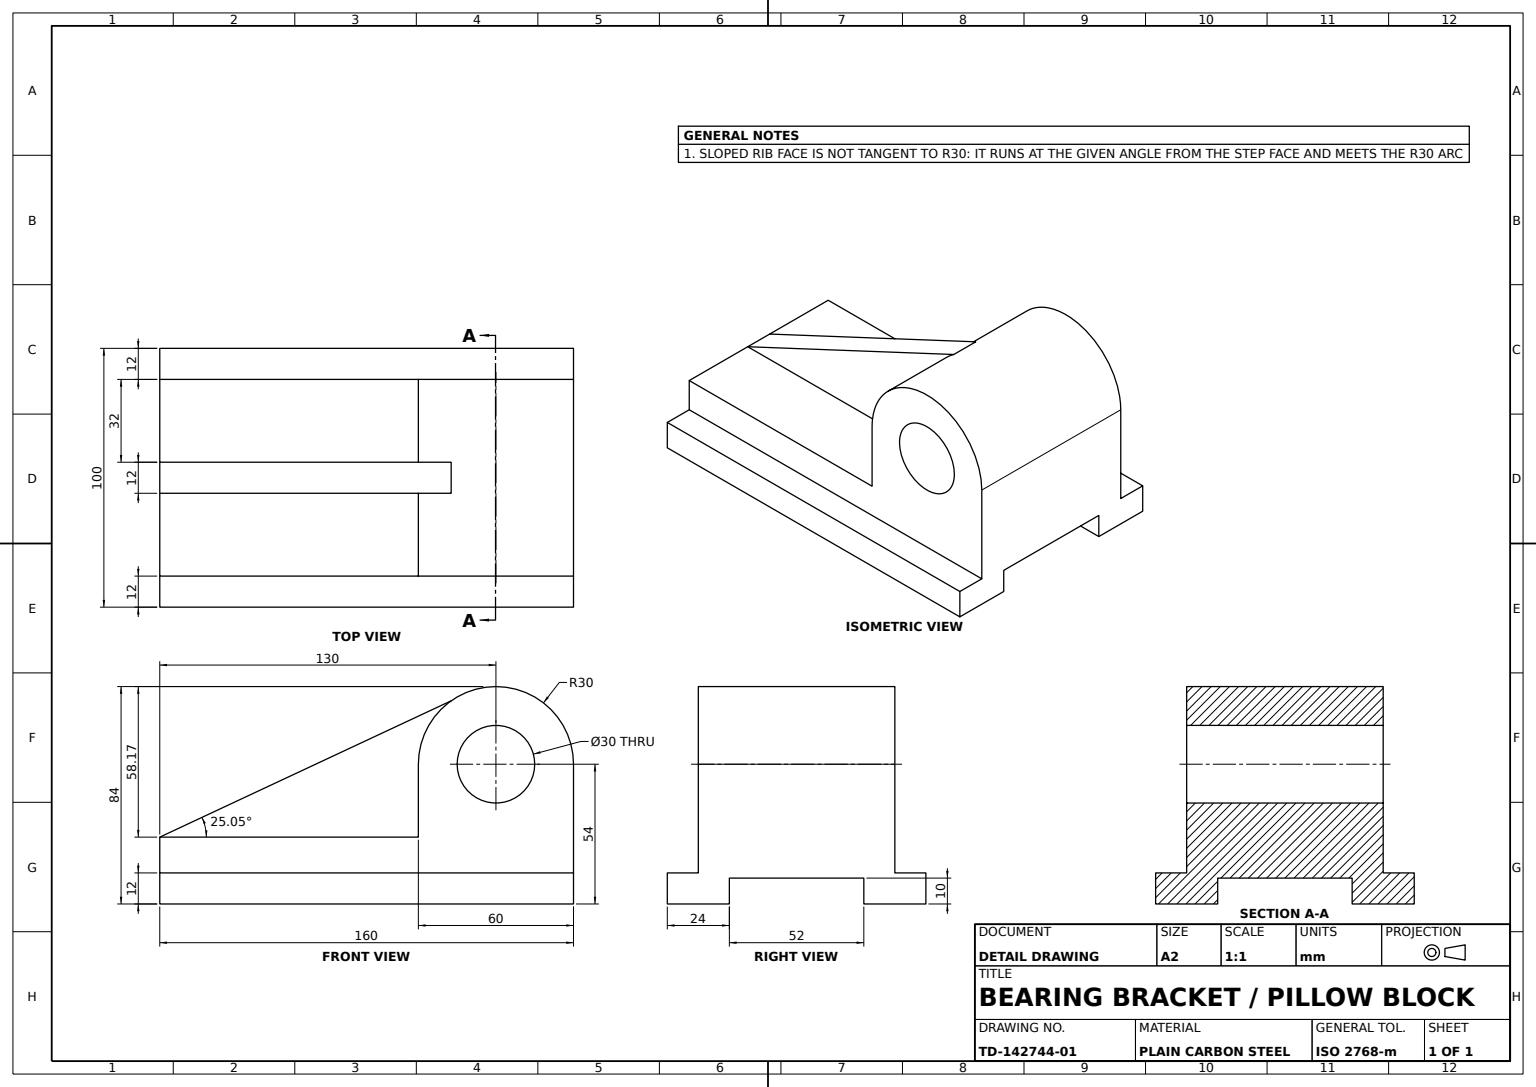
from build123d import *

# Parameters (mm, degrees)
BASE_SLIDE_PROFILE_SKETCH_W     = 76
BASE_SLIDE_PROFILE_SKETCH_H     = 60
BASE_BLOCK_160_DEPTH            = 160
BEARING_BLOCK_SHAPING_CUT_DEPTH = 198.027916804
SUPPORT_RIB_12_DEPTH            = 6
BORE_SKETCH_R                   = 15
BORE_30_DEPTH                   = 198.027916804


with BuildPart() as part:
    # Base Slide Profile Sketch → Base Block 160 (new body)
    with BuildSketch(Plane.XY):
        Polygon((-26, -10), (-26, 0), (26, 0), (26, -10), (50, -10), (50, 2), (38, 2), (38, 14), (-38, 14), (-38, 2), (-50, 2), (-50, -10), align=None)
        with Locations((0, 44)):
            Rectangle(BASE_SLIDE_PROFILE_SKETCH_W, BASE_SLIDE_PROFILE_SKETCH_H)
    extrude(amount=BASE_BLOCK_160_DEPTH)

    # Bearing Block Outline Sketch → Bearing Block Shaping Cut (cut, through all)
    with BuildSketch(Plane(origin=(38, 0, 0), x_dir=(0, 0, -1), z_dir=(1, 0, 0))):
        with BuildLine():
            Line((-60, 15.828860139), (-60, 44))
            ThreePointArc((-60, 44), (-51.213203403, 65.213203468), (-29.999999908, 74))
            Line((-29.999999908, 74), (-160, 74))
            Line((-160, 74), (-160, 15.828860139))
            Line((-160, 15.828860139), (-60, 15.828860139))
        make_face()
        with BuildLine():
            Line((0, 74), (-29.999999908, 74))
            ThreePointArc((-29.999999908, 74), (-8.786796532, 65.213203403), (0, 44))
            Line((0, 44), (0, 74))
        make_face()
    extrude(amount=-BEARING_BLOCK_SHAPING_CUT_DEPTH, mode=Mode.SUBTRACT)

    # Support Rib Sketch → Support Rib 12 (add, symmetric)
    with BuildSketch(Plane(origin=(0, 0, 0), x_dir=(0, 0, -1), z_dir=(1, 0, 0))):
        with BuildLine():
            Line((-160, 15.828860139), (-47.311623158, 68.501177597))
            ThreePointArc((-47.311623158, 68.501177597), (-56.639713725, 57.795856357), (-60, 44))
            Line((-60, 44), (-60, 15.828860139))
            Line((-60, 15.828860139), (-160, 15.828860139))
        make_face()
    extrude(amount=SUPPORT_RIB_12_DEPTH, both=True)

    # Bore Sketch → Bore Ø30 (cut, through all)
    with BuildSketch(Plane(origin=(38, 0, 0), x_dir=(0, 0, -1), z_dir=(1, 0, 0))):
        with Locations((-30, 44)):
            Circle(BORE_SKETCH_R)
    extrude(amount=-BORE_30_DEPTH, mode=Mode.SUBTRACT)


solid = part.part
